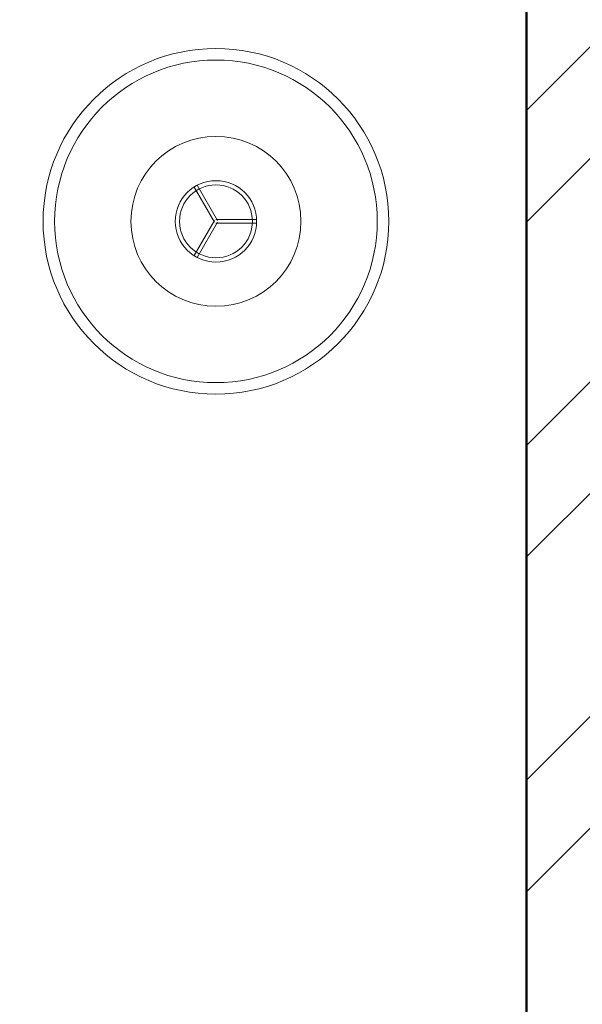
# Model space of a CAD drawing. Units: inches. Extents: x 963 to 2075, y 289 to 2657.
# Tile 72 of 98: x 1488 to 1511, y 2200 to 2239. Entities that reach past the tile are written whole.
import ezdxf

# ---------------------------------------------------------------- set-up
doc = ezdxf.new("R2010")
doc.units = ezdxf.units.IN
for name, color, linetype, lineweight in [('A-FURN', 8, 'Continuous', 18), ('A-WALL', 7, 'Continuous', 50), ('A-WALL-PATT', 8, 'Continuous', 13)]:
    doc.layers.add(name, color=color, linetype=linetype, lineweight=lineweight)

msp = doc.modelspace()

# ---------------------------------------------------------------- hatches: boundary and pattern name
at = {"layer": 'A-WALL-PATT'}
h = msp.add_hatch(dxfattribs=at)
h.set_pattern_fill('ANSI32', color=256)
h.paths.add_polyline_path([(1296.922, 2558.318), (1203.922, 2558.318), (1203.922, 2493.818), (1191.533, 2493.818), (1191.533, 2489.318), (1211.063, 2489.318), (1211.063, 2492.02), (1211.063, 2493.818), (1208.422, 2493.818), (1208.422, 2553.818), (1292.422, 2553.818), (1292.422, 2538.863), (1296.922, 2538.863)])
h.paths.add_polyline_path([(1442.422, 2558.318), (1349.422, 2558.318), (1349.422, 2538.943), (1353.922, 2538.943), (1353.922, 2553.818), (1437.922, 2553.818), (1437.922, 2493.818), (1434.542, 2493.818), (1434.542, 2489.318), (1448.311, 2489.318), (1448.311, 2491.568), (1448.311, 2493.818), (1442.422, 2493.818)])
h.paths.add_polyline_path([(1415.554, 2491.568), (1415.554, 2493.818), (1340.941, 2493.818), (1340.941, 2489.318), (1371.922, 2489.318), (1371.922, 2378.318), (1367.596, 2378.318), (1367.596, 2373.818), (1371.922, 2373.818), (1371.922, 2355.185), (1376.422, 2355.185), (1376.422, 2489.318), (1415.554, 2489.318)])
h.paths.add_polyline_path([(1304.941, 2491.568), (1304.941, 2493.818), (1296.922, 2493.818), (1296.922, 2514.863), (1292.422, 2514.863), (1292.422, 2493.818), (1232.808, 2493.818), (1232.808, 2489.318), (1256.422, 2489.318), (1256.422, 2327.318), (1253.714, 2327.318), (1253.714, 2322.818), (1328.422, 2322.818), (1328.422, 2331.147), (1323.922, 2331.147), (1323.922, 2327.318), (1260.922, 2327.318), (1260.922, 2373.818), (1323.922, 2373.818), (1323.922, 2357.812), (1328.422, 2357.812), (1328.422, 2373.818), (1346.007, 2373.818), (1346.007, 2376.068), (1346.007, 2378.318), (1260.922, 2378.318), (1260.922, 2489.318), (1304.941, 2489.318)])
h.paths.add_polyline_path([(1226.654, 2327.318), (1124.422, 2327.318), (1124.422, 2347.447), (1119.922, 2347.447), (1119.922, 2322.818), (1163.422, 2322.818), (1163.422, 2305.435), (1165.672, 2305.435), (1167.922, 2305.435), (1167.922, 2322.818), (1226.654, 2322.818), (1226.654, 2325.068)])
h.paths.add_polyline_path([(1095.922, 2489.318), (1124.422, 2489.318), (1131.533, 2489.318), (1131.533, 2491.568), (1131.533, 2493.818), (1119.922, 2493.818), (1091.422, 2493.818), (1091.422, 2417.318), (1095.922, 2417.318), (1119.922, 2417.318), (1119.922, 2407.447), (1124.422, 2407.447), (1124.422, 2421.818), (1095.922, 2421.818)])
h.paths.add_polyline_path([(1512.922, 2558.318), (1508.422, 2558.318), (1508.422, 2493.818), (1503.401, 2493.818), (1503.401, 2489.318), (1508.422, 2489.318), (1508.422, 2327.318), (1376.422, 2327.318), (1376.422, 2330.273), (1371.922, 2330.273), (1371.922, 2298.744), (1376.422, 2298.744), (1376.422, 2322.818), (1508.422, 2322.818), (1508.422, 2165.318), (1504.255, 2165.318), (1504.255, 2160.818), (1508.422, 2160.818), (1508.422, 2108.318), (1512.922, 2108.318), (1512.922, 2160.818), (1516.182, 2160.818), (1516.182, 2163.068), (1516.182, 2165.318), (1512.922, 2165.318), (1512.922, 2322.818), (1644.922, 2322.818), (1644.922, 2298.744), (1649.422, 2298.744), (1649.422, 2322.818), (1649.422, 2330.944), (1647.172, 2330.944), (1644.922, 2330.944), (1644.922, 2327.318), (1512.922, 2327.318), (1512.922, 2489.318), (1516.759, 2489.318), (1516.759, 2491.568), (1516.759, 2493.818), (1512.922, 2493.818)])
h.paths.add_polyline_path([(1671.922, 2558.318), (1578.922, 2558.318), (1578.922, 2493.818), (1573.526, 2493.818), (1573.526, 2489.318), (1586.537, 2489.318), (1586.537, 2491.568), (1586.537, 2493.818), (1583.422, 2493.818), (1583.422, 2553.818), (1667.422, 2553.818), (1667.422, 2541.109), (1671.922, 2541.109)])
h.paths.add_polyline_path([(1681.257, 2493.818), (1671.922, 2493.818), (1671.922, 2517.109), (1667.422, 2517.109), (1667.422, 2493.818), (1610.218, 2493.818), (1610.218, 2489.318), (1644.922, 2489.318), (1644.922, 2357.865), (1649.422, 2357.865), (1649.422, 2373.818), (1652.203, 2373.818), (1652.203, 2375.827), (1652.203, 2378.318), (1649.422, 2378.318), (1649.422, 2489.318), (1681.257, 2489.318), (1681.257, 2491.568)])
h.paths.add_polyline_path([(1821.922, 2558.318), (1728.922, 2558.318), (1728.922, 2541), (1733.422, 2541), (1733.422, 2553.818), (1817.422, 2553.818), (1817.422, 2493.818), (1813.507, 2493.818), (1813.507, 2489.318), (1830.078, 2489.318), (1830.078, 2491.568), (1830.078, 2493.818), (1821.922, 2493.818)])
h.paths.add_polyline_path([(1794.244, 2493.818), (1717.257, 2493.818), (1717.257, 2489.318), (1760.422, 2489.318), (1760.422, 2378.318), (1674.401, 2378.318), (1674.401, 2373.818), (1692.922, 2373.818), (1692.922, 2356.954), (1697.422, 2356.954), (1697.422, 2373.818), (1760.422, 2373.818), (1760.422, 2327.318), (1697.422, 2327.318), (1697.422, 2333.341), (1692.922, 2333.341), (1692.922, 2322.818), (1768.037, 2322.818), (1768.037, 2325.068), (1768.037, 2327.318), (1764.922, 2327.318), (1764.922, 2489.318), (1794.244, 2489.318)])
h.paths.add_polyline_path([(1733.422, 2517), (1728.922, 2517), (1728.922, 2493.818), (1733.422, 2493.818)], flags=17)
h.paths.add_polyline_path([(1929.922, 2493.818), (1890.078, 2493.818), (1890.078, 2489.318), (1896.922, 2489.318), (1925.422, 2489.318), (1925.422, 2421.818), (1896.922, 2421.818), (1896.922, 2408.318), (1901.422, 2408.318), (1901.422, 2417.318), (1925.422, 2417.318), (1929.922, 2417.318)])
h.paths.add_polyline_path([(1901.422, 2348.318), (1896.922, 2348.318), (1896.922, 2327.318), (1800.423, 2327.318), (1800.423, 2322.818), (1853.422, 2322.818), (1853.422, 2309.453), (1857.922, 2309.453), (1857.922, 2322.818), (1901.422, 2322.818)])
h.paths.add_polyline_path([(1857.922, 2249.453), (1853.422, 2249.453), (1853.422, 2214.818), (1686.309, 2214.818), (1686.309, 2210.318), (1853.422, 2210.318), (1853.422, 2202.134), (1857.922, 2202.134), (1857.922, 2210.318)])
h.paths.add_polyline_path([(1857.922, 2142.134), (1853.422, 2142.134), (1853.422, 2115.422), (1841.422, 2115.422), (1841.422, 2088.531), (1841.422, 2046.949), (1845.922, 2046.949), (1845.922, 2110.922), (1905.922, 2110.922), (1905.922, 2092.517), (1910.422, 2092.517), (1910.422, 2115.422), (1857.922, 2115.422)])
h.paths.add_polyline_path([(1532.436, 1482.342), (1573.456, 1482.342), (1573.456, 1501), (1532.436, 1501)], flags=9)
h.paths.add_polyline_path([(1438.658, 1486.302), (1479.678, 1486.302), (1479.678, 1504.96), (1438.658, 1504.96)], flags=9)
h.paths.add_polyline_path([(1411.215, 1365.308), (1659.139, 1365.308), (1659.139, 1402.401), (1411.215, 1402.401)], flags=9)
h.paths.add_polyline_path([(1185.671, 2296.298), (1248.16, 2296.298), (1248.16, 2314.955), (1185.671, 2314.955)], flags=9)
h.paths.add_polyline_path([(1177.31, 2187.35), (1216.15, 2187.35), (1216.15, 2206.007), (1177.31, 2206.007)], flags=9)
h.paths.add_polyline_path([(1295.101, 1602.083), (1328.26, 1602.083), (1328.26, 1620.741), (1295.101, 1620.741)], flags=9)
h.paths.add_polyline_path([(1525.126, 2005.99), (1558.39, 2005.99), (1558.39, 2024.648), (1525.126, 2024.648)], flags=9)
h.paths.add_polyline_path([(1459.606, 1977.125), (1472.195, 1977.125), (1472.195, 1987.429), (1459.606, 1987.429)], flags=9)
h.paths.add_polyline_path([(1467.815, 2053.676), (1480.018, 2053.676), (1480.018, 2063.979), (1467.815, 2063.979)], flags=9)
h.paths.add_polyline_path([(1555.184, 2119.02), (1584.563, 2119.02), (1584.563, 2137.678), (1555.184, 2137.678)], flags=25)
h.paths.add_polyline_path([(1405.389, 2115.291), (1444.478, 2115.291), (1444.478, 2133.948), (1405.389, 2133.948)], flags=25)
h.paths.add_polyline_path([(1698.482, 2004.259), (1727.695, 2004.259), (1727.695, 2022.916), (1698.482, 2022.916)], flags=9)
h.paths.add_polyline_path([(1612.158, 1972.855), (1629.016, 1972.855), (1629.016, 1983.159), (1612.158, 1983.159)], flags=9)
h.paths.add_polyline_path([(1608.289, 2060.036), (1625.147, 2060.036), (1625.147, 2070.34), (1608.289, 2070.34)], flags=9)
h.paths.add_polyline_path([(1527.954, 1684.402), (1566.795, 1684.402), (1566.795, 1703.06), (1527.954, 1703.06)], flags=9)
h.paths.add_polyline_path([(1422.792, 1683.59), (1461.633, 1683.59), (1461.633, 1702.247), (1422.792, 1702.247)], flags=9)
h.paths.add_polyline_path([(1531.262, 1732.459), (1574.015, 1732.459), (1574.015, 1751.116), (1531.262, 1751.116)], flags=9)
h.paths.add_polyline_path([(1402.872, 1732.845), (1439.799, 1732.845), (1439.799, 1751.502), (1402.872, 1751.502)], flags=9)
h.paths.add_polyline_path([(1243.122, 1923.132), (1281.962, 1923.132), (1281.962, 1941.79), (1243.122, 1941.79)], flags=9)
h.paths.add_polyline_path([(1181.752, 1792.268), (1244.241, 1792.268), (1244.241, 1810.926), (1181.752, 1810.926)], flags=9)
h.paths.add_polyline_path([(1265.822, 1670.3), (1316.071, 1670.3), (1316.071, 1688.957), (1265.822, 1688.957)], flags=9)
h.paths.add_polyline_path([(1140.263, 1676.054), (1179.104, 1676.054), (1179.104, 1694.711), (1140.263, 1694.711)], flags=9)
h.paths.add_polyline_path([(1107.49, 1490.889), (1143.374, 1490.889), (1143.374, 1509.546), (1107.49, 1509.546)], flags=9)
h.paths.add_polyline_path([(1217.584, 1483.899), (1246.741, 1483.899), (1246.741, 1502.556), (1217.584, 1502.556)], flags=9)
h.paths.add_polyline_path([(1389.21, 1486.919), (1418.367, 1486.919), (1418.367, 1505.576), (1389.21, 1505.576)], flags=9)
h.paths.add_polyline_path([(1672.208, 1602.083), (1705.366, 1602.083), (1705.366, 1620.741), (1672.208, 1620.741)], flags=9)
h.paths.add_polyline_path([(1752.082, 1522.638), (1781.24, 1522.638), (1781.24, 1541.295), (1752.082, 1541.295)], flags=9)
h.paths.add_polyline_path([(1848.275, 1491.26), (1884.158, 1491.26), (1884.158, 1509.918), (1848.275, 1509.918)], flags=9)
h.paths.add_polyline_path([(1822.47, 1685.62), (1861.31, 1685.62), (1861.31, 1704.278), (1822.47, 1704.278)], flags=9)
h.paths.add_polyline_path([(1713.195, 1672.232), (1763.444, 1672.232), (1763.444, 1690.889), (1713.195, 1690.889)], flags=9)
h.paths.add_polyline_path([(1736.619, 1790.578), (1799.109, 1790.578), (1799.109, 1809.235), (1736.619, 1809.235)], flags=9)
h.paths.add_polyline_path([(1691.491, 1916.355), (1730.332, 1916.355), (1730.332, 1935.013), (1691.491, 1935.013)], flags=9)
h.paths.add_polyline_path([(1764.872, 1973.922), (1794.306, 1973.922), (1794.306, 1992.58), (1764.872, 1992.58)], flags=9)
h.paths.add_polyline_path([(1767.854, 2034.017), (1797.288, 2034.017), (1797.288, 2052.674), (1767.854, 2052.674)], flags=9)
h.paths.add_polyline_path([(1851.593, 2060.331), (1880.751, 2060.331), (1880.751, 2078.989), (1851.593, 2078.989)], flags=25)
h.paths.add_polyline_path([(1688.491, 2086.874), (1727.332, 2086.874), (1727.332, 2105.531), (1688.491, 2105.531)], flags=9)
h.paths.add_polyline_path([(1537.743, 2293.581), (1580.495, 2293.581), (1580.495, 2312.239), (1537.743, 2312.239)], flags=25)
h.paths.add_polyline_path([(1425.587, 2296.109), (1468.34, 2296.109), (1468.34, 2314.766), (1425.587, 2314.766)], flags=25)
h.paths.add_polyline_path([(1278.518, 2004.184), (1307.72, 2004.184), (1307.72, 2022.841), (1278.518, 2022.841)], flags=9)
h.paths.add_polyline_path([(1193.282, 1973.635), (1222.715, 1973.635), (1222.715, 1992.292), (1193.282, 1992.292)], flags=9)
h.paths.add_polyline_path([(1192.411, 2040.577), (1221.845, 2040.577), (1221.845, 2059.234), (1192.411, 2059.234)], flags=9)
h.paths.add_polyline_path([(1130.603, 1951.393), (1159.76, 1951.393), (1159.76, 1970.05), (1130.603, 1970.05)], flags=9)
h.paths.add_polyline_path([(1132.827, 2052.494), (1161.984, 2052.494), (1161.984, 2071.151), (1132.827, 2071.151)], flags=9)
h.paths.add_polyline_path([(1265.128, 2334.619), (1315.377, 2334.619), (1315.377, 2353.277), (1265.128, 2353.277)], flags=25)
h.paths.add_polyline_path([(1136.741, 2330.785), (1175.582, 2330.785), (1175.582, 2349.443), (1136.741, 2349.443)], flags=9)
h.paths.add_polyline_path([(1287.422, 2417.204), (1320.58, 2417.204), (1320.58, 2435.861), (1287.422, 2435.861)], flags=25)
h.paths.add_polyline_path([(1430.988, 2329.159), (1469.828, 2329.159), (1469.828, 2347.816), (1430.988, 2347.816)], flags=25)
h.paths.add_polyline_path([(1525.424, 2329.213), (1564.264, 2329.213), (1564.264, 2347.87), (1525.424, 2347.87)], flags=25)
h.paths.add_polyline_path([(1684.525, 2382.799), (1717.683, 2382.799), (1717.683, 2401.457), (1684.525, 2401.457)], flags=25)
h.paths.add_polyline_path([(1704.805, 2340.293), (1755.054, 2340.293), (1755.054, 2358.95), (1704.805, 2358.95)], flags=25)
h.paths.add_polyline_path([(1694.113, 2287.757), (1756.602, 2287.757), (1756.602, 2306.414), (1694.113, 2306.414)], flags=9)
h.paths.add_polyline_path([(1815.778, 2329.861), (1854.618, 2329.861), (1854.618, 2348.518), (1815.778, 2348.518)], flags=9)
h.paths.add_polyline_path([(1842.873, 2514.256), (1878.756, 2514.256), (1878.756, 2532.914), (1842.873, 2532.914)], flags=9)
h.paths.add_polyline_path([(1769.513, 2531.447), (1798.671, 2531.447), (1798.671, 2550.104), (1769.513, 2550.104)], flags=25)
h.paths.add_polyline_path([(1594.772, 2518.468), (1623.93, 2518.468), (1623.93, 2537.125), (1594.772, 2537.125)], flags=25)
h.paths.add_polyline_path([(1520.723, 2516.185), (1556.606, 2516.185), (1556.606, 2534.842), (1520.723, 2534.842)], flags=25)
h.paths.add_polyline_path([(1464.456, 2516.694), (1500.34, 2516.694), (1500.34, 2535.351), (1464.456, 2535.351)], flags=25)
h.paths.add_polyline_path([(1365.696, 2528.97), (1394.854, 2528.97), (1394.854, 2547.627), (1365.696, 2547.627)], flags=25)
h.paths.add_polyline_path([(1222.838, 2516.231), (1251.995, 2516.231), (1251.995, 2534.889), (1222.838, 2534.889)], flags=25)
h.paths.add_polyline_path([(1104.545, 2509.6), (1140.429, 2509.6), (1140.429, 2528.257), (1104.545, 2528.257)], flags=9)

# ---------------------------------------------------------------- linework, layer by layer
at = {"layer": 'A-FURN', "ltscale": 0.03}
for p, q in [((1495.872, 2231.329), (1495.055, 2232.744)), ((1495.998, 2231.402), (1495.181, 2232.817)), ((1495.872, 2231.402), (1495.055, 2229.987)), ((1495.998, 2231.329), (1495.181, 2229.914)), ((1495.935, 2231.438), (1497.569, 2231.438)), ((1495.935, 2231.292), (1497.569, 2231.292))]:
    msp.add_line(p, q, dxfattribs=at)
for radius in [6.953, 3.418, 1.636, 1.466]:
    msp.add_circle((1495.935, 2231.365), radius, dxfattribs=at)
at = {"layer": 'A-FURN'}
msp.add_circle((1495.935, 2231.365), 6.489, dxfattribs=at)
at = {"layer": 'A-WALL'}
msp.add_line((1508.422, 2322.818), (1508.422, 2165.318), dxfattribs=at)

doc.saveas('drawing.dxf')
